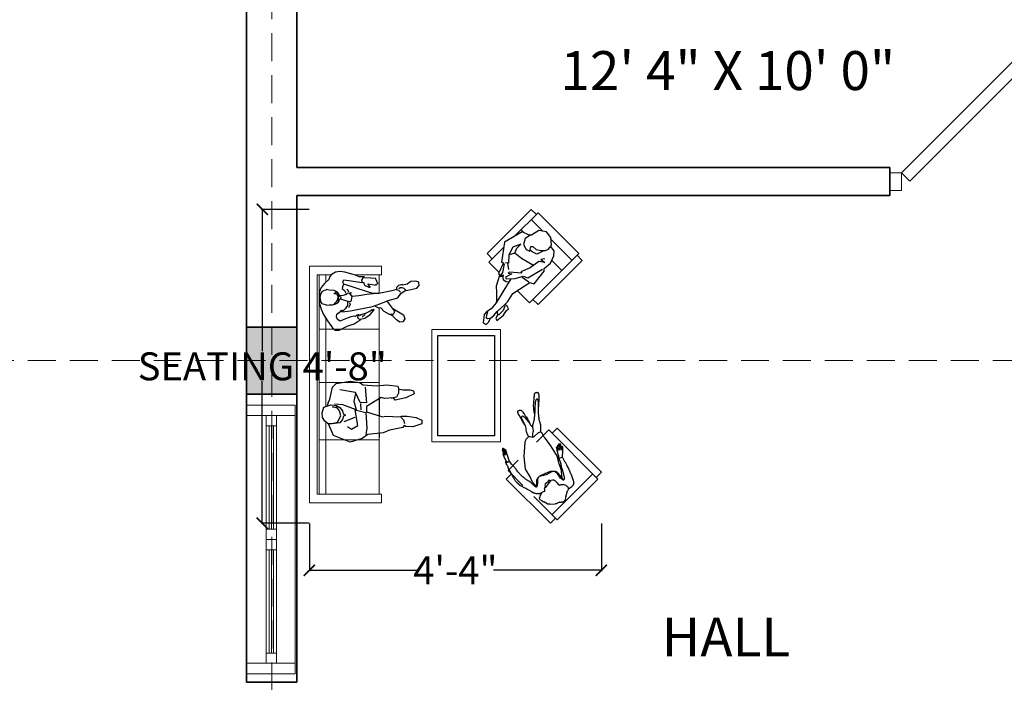
# Model space of a CAD drawing. Units: inches. Extents: x 782 to 2660, y -1008 to 166.
# Tile 7 of 12: x 1058 to 1234, y -176 to -58. Entities that reach past the tile are written whole.
import ezdxf

# ---------------------------------------------------------------- set-up
doc = ezdxf.new("R2010")
doc.units = ezdxf.units.IN
doc.header["$MEASUREMENT"] = 0
doc.linetypes.add('DASHED', pattern=[0.75, 0.5, -0.25])
for name, color, linetype, lineweight in [('A-ANNO-DIMS', 4, 'Continuous', 18), ('A-AREA-IDEN', 4, 'Continuous', 18), ('A-COLS', 7, 'Continuous', 35), ('A-Door', 150, 'Continuous', 18), ('A-FURN', 8, 'Continuous', 13), ('A-Glaz', 4, 'Continuous', 18), ('A-GRID', 8, 'DASHED', 13), ('A-WALL', 7, 'Continuous', 35)]:
    doc.layers.add(name, color=color, linetype=linetype, lineweight=lineweight)
doc.layers.add('NET 01', color=8, linetype='Continuous')
doc.layers.add('NOITHAT', color=21, linetype='Continuous')
doc.styles.get("Standard").update_dxf_attribs({"font": 'arial.ttf'})
doc.dimstyles.get("Standard").update_dxf_attribs({"dimtxt": 5, "dimasz": 2, "dimexe": 0.18, "dimexo": 0.0625, "dimgap": 0.09, "dimtad": 0, "dimtih": 1, "dimtoh": 1, "dimdec": 0, "dimzin": 0, "dimdsep": 46, "dimlunit": 3, "dimtxsty": 'Standard', "dimblk": 'ARCHTICK', "dimcen": 0.09, "dimadec": 0, "dimazin": 0, "dimtfac": 1, "dimtdec": 0, "dimtofl": 0, "dimtmove": 0, "dimatfit": 3, "dimfxl": 1, "dimtolj": 1, "dimtzin": 0, "dimarcsym": 0})

# ---------------------------------------------------------------- blocks, each defined once
blk = doc.blocks.new('A$C592222DF')
at = {"layer": 'A-Door'}
for points in [[(-0.0354, -0.0354), (-0.6718, 0.601), (-0.6364, 0.6364), (0, 0)], [(-0.95, 0), (-0.95, -0.075), (-0.9, -0.075), (-0.9, 0)], [(0, 0), (0, -0.075), (0.05, -0.075), (0.05, 0)]]:
    blk.add_lwpolyline(points, close=True, dxfattribs=at)
at = {"layer": 'NET 01'}
blk.add_arc((0, 0), 0.9, 135, 180, dxfattribs=at)
blk = doc.blocks.new('02PFMA09')
at = {"color": 0, "linetype": 'ByBlock'}
for p, q in [((3.05, 8.92), (3.14, 9)), ((3.13, 7.43), (3.05, 8.92)), ((3.14, 9), (3.16, 8.93)), ((5.73, 9.76), (5.71, 9.77)), ((5.73, 9.76), (5.72, 9.77)), ((-13.1, 3.75), (-12.15, 4.37)), ((-12.31, 4.26), (-10.34, 5.72)), ((-10.32, 5.71), (-10.21, 5.9)), ((-9.79, 6.26), (-10.21, 5.9)), ((-9.79, 6.35), (-9.8, 6.25)), ((-8.24, 6.17), (-8.66, 6.39)), ((-8.12, 6.08), (-8.24, 6.17)), ((-8.12, 6.08), (-7.24, 4.99)), ((-7.02, 3.76), (-7.02, 4.36)), ((-4.78, 5.75), (-5.53, 5.7)), ((-4.02, 5.38), (-5.5, 5.67)), ((-4.78, 5.75), (-2.07, 6.47)), ((-2.3, 4.9), (-4.02, 5.38)), ((-2.4, 4.61), (-1.25, 4.02)), ((-2.3, 4.9), (-2.23, 4.9)), ((0.87, 6.65), (-2.07, 6.47)), ((-1.29, 4.26), (-1.18, 3.98)), ((0.87, 6.65), (3.72, 7.15)), ((3.13, 7.43), (3.55, 7.64)), ((3.55, 7.64), (3.51, 7.76)), ((9.01, 6.24), (4.07, 7.14)), ((13.28, 5.24), (9.01, 6.24)), ((13.28, 5.24), (15.05, 5.1)), ((15.45, 4.82), (15.72, 4.28)), ((15.49, 4.74), (18.19, 5.91)), ((18.19, 5.91), (20.99, 6.15)), ((21.57, 4.27), (19.72, 2.97)), ((23.19, 6.75), (20.99, 6.15)), ((23.07, 5.07), (21.57, 4.27)), ((23.85, 5.5), (23.07, 5.07)), ((24.19, 7.17), (23.19, 6.75)), ((24.19, 7.17), (24.32, 7.29)), ((-13.7, 2), (-13.76, 2.21)), ((-13.66, 2.99), (-13.41, 3.42)), ((-13.36, 1.1), (-13.36, -0.48)), ((-6.7, 3.3), (-6.6, 3.26)), ((-5.84, 3.17), (-6.6, 3.26)), ((-5.84, 3.17), (-5.39, 2.98)), ((-4.55, 2.65), (-5.39, 2.98)), ((-4.85, -0.2), (-3.86, 1.35)), ((-4.08, 0.8), (-4.09, 0.98)), ((-3.5, 0.53), (-4.08, 0.8)), ((-3.5, 0.16), (-4.08, -0.2)), ((-3.86, 1.35), (-3.92, 1.85)), ((-3.5, 0.53), (-3.5, 0.16)), ((-0.77, 3.02), (-1.15, 0.28)), ((-1.15, 0.28), (-0.77, -2.45)), ((-0.6, 2.93), (-0.76, 3.23)), ((-0.48, -1.9), (-0.48, 2.46)), ((14.87, 1.49), (15.75, 3.89)), ((15.65, 0.15), (14.96, 1)), ((15.04, 0.89), (15.44, 1.22)), ((15.44, 1.22), (16.2, 1.52)), ((16.2, 1.52), (16.89, 2)), ((18.39, 2.4), (16.89, 2)), ((18.39, 2.4), (19.72, 2.97)), ((20.04, 0.06), (20.17, 0.06)), ((20.17, 0.06), (20.79, -0.03)), ((-12.58, -2.84), (-13.3, -0.82)), ((-12.58, -2.84), (-12.41, -3.29)), ((-12.07, -3.74), (-10.72, -4.74)), ((-7, -3.4), (-7.02, -4.02)), ((-6.6, -2.66), (-6.77, -2.66)), ((-6.03, -2.48), (-6.6, -2.66)), ((-6.03, -2.48), (-5.6, -2.2)), ((-5.6, -2.2), (-5.44, -1.42)), ((-5.29, -1.93), (-5.55, -1.94)), ((-5.44, -1.42), (-4.85, -0.2)), ((-4.71, -1.75), (-5.29, -1.93)), ((-4.34, -1.47), (-4.71, -1.75)), ((-4.08, -0.2), (-4.34, -1.47)), ((-1.19, -3.54), (-1.1, -3.36)), ((-0.73, -2.64), (-0.59, -2.36)), ((9.01, -5.17), (14.26, -2.61)), ((14.4, -2.51), (15.2, -1.7)), ((15.73, -0.33), (15.32, -1.51)), ((-10.25, -5.27), (-10.43, -5.08)), ((-10.21, -5.2), (-10.25, -5.27)), ((-9.79, -5.57), (-10.21, -5.2)), ((-8.24, -5.48), (-8.66, -5.7)), ((-8.12, -5.39), (-8.24, -5.48)), ((-7.02, -4.02), (-8.12, -5.39)), ((-2.07, -5.87), (-4.12, -5.33)), ((-3.98, -5.05), (-4.11, -5.05)), ((-3.98, -5.05), (-2.34, -4.32)), ((-2.34, -4.32), (-1.65, -3.99)), ((-2.07, -5.87), (0.87, -6.06)), ((0.87, -6.06), (3.67, -6.54)), ((4.11, -6.52), (9.01, -5.17)), ((12.6, -12.12), (12.56, -12.13))]:
    blk.add_line(p, q, dxfattribs=at)
blk.add_line((0, 0), (0, 0))
for points in [[(3.14, 9), (2.51, 9.01), (2.01, 9.04), (1.62, 9.06), (1.33, 9.1), (1.12, 9.13), (0.97, 9.16), (0.87, 9.2), (0.79, 9.23), (0.73, 9.25), (0.67, 9.28), (0.6, 9.3), (0.5, 9.31), (0.37, 9.33), (0.19, 9.35), (-0.05, 9.36), (-0.35, 9.38), (-0.73, 9.41), (-1.17, 9.43), (-1.65, 9.46), (-2.15, 9.49), (-2.66, 9.51), (-3.14, 9.54), (-3.59, 9.56), (-3.97, 9.57), (-4.29, 9.59), (-4.53, 9.6), (-4.72, 9.6), (-4.87, 9.6), (-4.98, 9.6), (-5.08, 9.6), (-5.16, 9.59), (-5.25, 9.59), (-5.35, 9.58), (-5.45, 9.57), (-5.57, 9.56), (-5.69, 9.55), (-5.82, 9.54), (-5.94, 9.54), (-6.06, 9.53), (-6.18, 9.52), (-6.29, 9.51), (-6.39, 9.51), (-6.48, 9.5), (-6.56, 9.5), (-6.64, 9.5), (-6.7, 9.49), (-6.76, 9.49), (-6.81, 9.49), (-6.86, 9.49), (-6.89, 9.49), (-6.93, 9.49), (-6.96, 9.49), (-7, 9.49), (-7.05, 9.48), (-7.1, 9.48), (-7.16, 9.47), (-7.24, 9.46), (-7.32, 9.45), (-7.42, 9.44), (-7.51, 9.43), (-7.61, 9.42), (-7.7, 9.4), (-7.79, 9.39), (-7.87, 9.38), (-7.93, 9.37), (-7.99, 9.36), (-8.03, 9.35), (-8.07, 9.34), (-8.11, 9.33), (-8.14, 9.32), (-8.17, 9.31), (-8.21, 9.3), (-8.25, 9.29), (-8.3, 9.27), (-8.35, 9.25), (-8.42, 9.22), (-8.49, 9.18), (-8.57, 9.12), (-8.66, 9.05), (-8.77, 8.97), (-8.89, 8.86), (-9.02, 8.72), (-9.16, 8.53), (-9.3, 8.27), (-9.43, 7.94), (-9.56, 7.52), (-9.68, 6.99), (-9.79, 6.35)], [(5.68, 9.76), (5.96, 9.86), (6.2, 9.95), (6.4, 10.04), (6.57, 10.11), (6.71, 10.18), (6.83, 10.24), (6.92, 10.29), (6.99, 10.34), (7.03, 10.38), (7.07, 10.41), (7.09, 10.44), (7.09, 10.47), (7.09, 10.49), (7.08, 10.5), (7.06, 10.52), (7.04, 10.53), (7.01, 10.54), (6.99, 10.55), (6.95, 10.55), (6.9, 10.55), (6.83, 10.54), (6.74, 10.52), (6.63, 10.49), (6.49, 10.45), (6.32, 10.4), (6.13, 10.34), (5.91, 10.27), (5.69, 10.19), (5.46, 10.1), (5.22, 10.01), (5, 9.91), (4.79, 9.8), (4.59, 9.7), (4.41, 9.59), (4.23, 9.48), (4.04, 9.36), (3.84, 9.25), (3.61, 9.13), (3.35, 9.01), (3.05, 8.89)], [(3.12, 7.71), (3.95, 7.81), (4.67, 7.89), (5.29, 7.97), (5.81, 8.04), (6.25, 8.1), (6.61, 8.15), (6.9, 8.2), (7.14, 8.25), (7.32, 8.29), (7.47, 8.33), (7.57, 8.36), (7.65, 8.4), (7.69, 8.43), (7.72, 8.46), (7.73, 8.49), (7.73, 8.52), (7.72, 8.55), (7.7, 8.57), (7.65, 8.59), (7.56, 8.62), (7.43, 8.63), (7.25, 8.65), (7, 8.66), (6.68, 8.66)], [(6.02, 8.53), (6.72, 8.67), (7.25, 8.79), (7.63, 8.89), (7.88, 8.96), (8.03, 9.02), (8.1, 9.07), (8.12, 9.11), (8.12, 9.15), (8.1, 9.18), (8.08, 9.2), (8.04, 9.23), (7.97, 9.25), (7.87, 9.26), (7.73, 9.26), (7.54, 9.25), (7.3, 9.23)], [(7.19, 9.74), (7.59, 9.77), (7.9, 9.78), (8.12, 9.78), (8.28, 9.77), (8.38, 9.76), (8.44, 9.74), (8.47, 9.71), (8.49, 9.68), (8.49, 9.64), (8.46, 9.6), (8.38, 9.55), (8.2, 9.48), (7.91, 9.39), (7.47, 9.28), (6.86, 9.14), (6.05, 8.97)], [(6.49, 10.05), (7.06, 10.13), (7.49, 10.19), (7.8, 10.22), (8.02, 10.24), (8.16, 10.23), (8.24, 10.22), (8.28, 10.19), (8.29, 10.16), (8.3, 10.13), (8.27, 10.09), (8.19, 10.04), (8.04, 9.97), (7.77, 9.89), (7.37, 9.79), (6.82, 9.67), (6.08, 9.51)], [(23.49, 5.3), (23.63, 5.3), (23.83, 5.32), (24.11, 5.37), (24.43, 5.44), (24.81, 5.53), (25.24, 5.66), (25.7, 5.81), (26.19, 5.99), (26.71, 6.21), (27.25, 6.45), (27.78, 6.7), (28.3, 6.96), (28.8, 7.22), (29.26, 7.46), (29.68, 7.68), (30.03, 7.88), (30.31, 8.03), (30.52, 8.15), (30.68, 8.25), (30.8, 8.32), (30.87, 8.38), (30.92, 8.42), (30.95, 8.46), (30.97, 8.51), (30.99, 8.56), (31, 8.62), (31.02, 8.68), (31.03, 8.75), (31.04, 8.82), (31.05, 8.9), (31.05, 8.98), (31.05, 9.06), (31.05, 9.14), (31.04, 9.22), (31.02, 9.3), (31, 9.38), (30.97, 9.45), (30.93, 9.52), (30.88, 9.58), (30.82, 9.64), (30.75, 9.69), (30.67, 9.73), (30.58, 9.76), (30.47, 9.77), (30.36, 9.78), (30.23, 9.78), (30.1, 9.77), (29.95, 9.74), (29.78, 9.7), (29.57, 9.64), (29.27, 9.52), (28.86, 9.35), (28.29, 9.1), (27.53, 8.76), (26.55, 8.31), (25.31, 7.73)], [(24.32, 7.29), (25.49, 7.8), (26.4, 8.17), (27.09, 8.42), (27.59, 8.56), (27.94, 8.62), (28.17, 8.61), (28.31, 8.56), (28.39, 8.48), (28.45, 8.38), (28.48, 8.28), (28.47, 8.17), (28.43, 8.05), (28.34, 7.91), (28.2, 7.76), (28.01, 7.6), (27.77, 7.42), (27.46, 7.22), (27.08, 7.01), (26.66, 6.78), (26.18, 6.54), (25.66, 6.29), (25.09, 6.04), (24.48, 5.77), (23.85, 5.5)], [(20.79, -0.03), (22.71, -0.38), (24.15, -0.61), (25.2, -0.75), (25.92, -0.81), (26.37, -0.82), (26.62, -0.77), (26.73, -0.7), (26.78, -0.63), (26.82, -0.56), (26.85, -0.5), (26.88, -0.45), (26.91, -0.4), (26.94, -0.35), (26.96, -0.29), (26.97, -0.23), (26.98, -0.17), (26.98, -0.09), (26.98, -0.01), (26.96, 0.08), (26.95, 0.17), (26.93, 0.27), (26.9, 0.36), (26.88, 0.45), (26.85, 0.54), (26.82, 0.62), (26.78, 0.69), (26.7, 0.77), (26.57, 0.84), (26.39, 0.92), (26.12, 1.01), (25.77, 1.11), (25.3, 1.23), (24.72, 1.36), (24.05, 1.5), (23.31, 1.64), (22.54, 1.76), (21.77, 1.87), (21.02, 1.96), (20.33, 2), (19.74, 2.01)], [(20.17, 0.06), (21.44, -0.08), (22.42, -0.16), (23.16, -0.19), (23.69, -0.17), (24.04, -0.11), (24.25, -0.02), (24.36, 0.09), (24.4, 0.22), (24.41, 0.36), (24.34, 0.5), (24.16, 0.67), (23.83, 0.86), (23.3, 1.09), (22.54, 1.35), (21.5, 1.66), (20.21, 2)], [(-1.25, -3.45), (-1.62, -3.66), (-1.92, -3.82), (-2.16, -3.95), (-2.36, -4.05), (-2.52, -4.12), (-2.66, -4.18), (-2.79, -4.23), (-2.93, -4.29), (-3.08, -4.36), (-3.24, -4.44), (-3.4, -4.53), (-3.56, -4.62), (-3.72, -4.71), (-3.86, -4.81), (-3.98, -4.91), (-4.07, -5), (-4.13, -5.09), (-4.16, -5.17), (-4.15, -5.25), (-4.12, -5.33), (-4.06, -5.41), (-3.96, -5.49), (-3.84, -5.57), (-3.69, -5.66), (-3.51, -5.74), (-3.3, -5.84), (-3.08, -5.94), (-2.83, -6.05), (-2.57, -6.16), (-2.3, -6.29), (-2.02, -6.43), (-1.74, -6.58), (-1.45, -6.75), (-1.17, -6.93), (-0.89, -7.11), (-0.62, -7.3), (-0.37, -7.47), (-0.13, -7.64), (0.08, -7.79), (0.28, -7.92), (0.44, -8.03), (0.58, -8.11), (0.7, -8.17), (0.8, -8.22), (0.88, -8.26), (0.95, -8.29), (1.01, -8.32), (1.07, -8.34), (1.12, -8.37), (1.17, -8.4), (1.22, -8.44), (1.29, -8.49), (1.37, -8.54), (1.47, -8.6), (1.59, -8.67), (1.74, -8.76), (1.93, -8.85), (2.14, -8.96), (2.38, -9.07), (2.65, -9.19), (2.95, -9.32), (3.27, -9.44), (3.61, -9.56), (3.97, -9.68), (4.35, -9.79), (4.74, -9.9), (5.14, -10), (5.53, -10.09), (5.91, -10.19), (6.27, -10.28), (6.6, -10.38), (6.9, -10.48), (7.16, -10.58), (7.4, -10.69), (7.64, -10.8), (7.91, -10.91), (8.21, -11.02), (8.58, -11.12), (9.04, -11.23), (9.6, -11.34)], [(-7.02, -4.02), (-7.07, -4.21), (-7.11, -4.36), (-7.13, -4.47), (-7.15, -4.55), (-7.15, -4.62), (-7.15, -4.68), (-7.15, -4.75), (-7.15, -4.82), (-7.14, -4.91), (-7.13, -5.01), (-7.12, -5.13), (-7.1, -5.26), (-7.07, -5.4), (-7.03, -5.55), (-6.98, -5.71), (-6.91, -5.87), (-6.82, -6.04), (-6.72, -6.21), (-6.6, -6.37), (-6.48, -6.53), (-6.36, -6.68), (-6.23, -6.83), (-6.11, -6.97), (-5.99, -7.09), (-5.89, -7.2), (-5.78, -7.3), (-5.68, -7.39), (-5.58, -7.48), (-5.47, -7.57), (-5.35, -7.67), (-5.21, -7.78), (-5.05, -7.89), (-4.87, -8.03), (-4.67, -8.18), (-4.45, -8.34), (-4.21, -8.52), (-3.96, -8.71), (-3.7, -8.92), (-3.43, -9.13), (-3.15, -9.35), (-2.88, -9.58), (-2.6, -9.82), (-2.33, -10.05), (-2.07, -10.27), (-1.82, -10.49), (-1.59, -10.68), (-1.38, -10.85), (-1.19, -10.99), (-1.03, -11.11), (-0.89, -11.19), (-0.78, -11.25), (-0.68, -11.29), (-0.59, -11.32), (-0.51, -11.34), (-0.42, -11.36), (-0.34, -11.39), (-0.25, -11.42), (-0.15, -11.47), (-0.05, -11.51), (0.06, -11.57), (0.18, -11.63), (0.3, -11.69), (0.43, -11.75), (0.57, -11.81), (0.71, -11.87), (0.86, -11.93), (1.03, -11.98), (1.22, -12.04), (1.45, -12.09), (1.7, -12.15), (2, -12.2), (2.35, -12.25), (2.74, -12.3), (3.17, -12.35), (3.63, -12.4), (4.09, -12.45), (4.55, -12.49), (4.99, -12.53), (5.4, -12.57), (5.77, -12.61), (6.08, -12.64), (6.33, -12.67), (6.54, -12.7), (6.7, -12.72), (6.84, -12.74), (6.95, -12.75), (7.04, -12.76), (7.13, -12.76), (7.2, -12.76), (7.28, -12.76), (7.35, -12.75), (7.42, -12.74), (7.49, -12.73), (7.55, -12.72), (7.62, -12.71), (7.69, -12.7), (7.75, -12.7), (7.84, -12.7), (7.97, -12.71), (8.15, -12.72), (8.4, -12.75), (8.75, -12.79), (9.21, -12.84), (9.8, -12.91)], [(10, -12.41), (9.95, -12.7), (9.89, -12.86), (9.81, -12.9), (9.74, -12.85), (9.67, -12.74), (9.61, -12.57), (9.56, -12.38), (9.53, -12.18), (9.51, -12), (9.52, -11.84), (9.54, -11.7), (9.57, -11.58), (9.6, -11.49), (9.63, -11.41), (9.65, -11.37), (9.66, -11.35)], [(12.73, -11.52), (13.36, -11.44), (13.82, -11.38), (14.16, -11.33), (14.38, -11.3), (14.51, -11.27), (14.57, -11.24), (14.59, -11.22), (14.59, -11.21), (14.58, -11.19), (14.58, -11.17), (14.57, -11.15), (14.57, -11.13), (14.56, -11.12), (14.55, -11.1), (14.54, -11.09), (14.53, -11.07), (14.51, -11.06), (14.48, -11.06), (14.44, -11.05), (14.39, -11.05), (14.32, -11.05), (14.23, -11.06), (14.12, -11.06), (13.98, -11.07), (13.82, -11.09), (13.62, -11.1), (13.41, -11.12), (13.19, -11.14), (12.95, -11.16), (12.71, -11.18), (12.47, -11.2), (12.24, -11.22), (12.03, -11.25), (11.82, -11.27), (11.63, -11.29), (11.44, -11.31), (11.27, -11.33), (11.12, -11.34), (10.97, -11.35), (10.84, -11.36), (10.71, -11.36), (10.6, -11.37), (10.48, -11.37), (10.35, -11.37), (10.2, -11.38), (10.04, -11.4), (9.84, -11.42), (9.61, -11.46)], [(14.99, -11.92), (15.09, -11.9), (15.17, -11.88), (15.23, -11.85), (15.27, -11.83), (15.3, -11.8), (15.32, -11.77), (15.32, -11.74), (15.32, -11.71), (15.32, -11.67), (15.28, -11.64), (15.18, -11.62), (14.99, -11.61), (14.67, -11.61), (14.2, -11.64), (13.54, -11.7), (12.67, -11.79)], [(14.99, -11.54), (14.99, -11.51), (14.96, -11.47), (14.88, -11.43), (14.71, -11.4), (14.44, -11.39), (14.04, -11.4), (13.48, -11.44), (12.73, -11.52)], [(9.56, -12.39), (9.77, -12.4), (9.94, -12.41), (10.08, -12.42), (10.2, -12.44), (10.3, -12.45), (10.39, -12.47), (10.46, -12.48), (10.52, -12.49), (10.58, -12.5), (10.64, -12.51), (10.7, -12.51), (10.76, -12.52), (10.82, -12.53), (10.89, -12.53), (10.97, -12.54), (11.05, -12.54), (11.13, -12.55), (11.23, -12.56), (11.33, -12.58), (11.43, -12.59), (11.52, -12.6), (11.61, -12.61), (11.7, -12.62), (11.77, -12.62), (11.83, -12.62), (11.89, -12.62), (11.93, -12.62), (11.97, -12.62), (12.01, -12.61), (12.05, -12.61), (12.1, -12.6), (12.14, -12.6), (12.2, -12.59), (12.27, -12.59), (12.34, -12.59), (12.41, -12.58), (12.48, -12.58), (12.55, -12.58), (12.61, -12.58), (12.67, -12.59), (12.73, -12.59), (12.77, -12.59), (12.81, -12.59), (12.85, -12.6), (12.88, -12.6), (12.92, -12.6), (12.95, -12.61), (12.99, -12.61), (13.03, -12.62), (13.07, -12.62), (13.11, -12.62), (13.15, -12.62), (13.18, -12.61), (13.21, -12.6), (13.23, -12.59), (13.24, -12.56), (13.24, -12.53), (13.21, -12.49), (13.17, -12.45), (13.11, -12.39), (13.02, -12.34), (12.89, -12.27), (12.74, -12.2), (12.54, -12.13)], [(13.04, -12.35), (13.55, -12.31), (14.08, -12.26), (14.46, -12.21), (14.72, -12.18), (14.87, -12.14), (14.95, -12.11), (14.98, -12.08), (14.99, -12.04), (14.98, -12.01), (14.95, -11.98), (14.86, -11.96), (14.69, -11.94), (14.4, -11.95), (13.98, -11.98), (13.38, -12.03), (12.6, -12.12)]]:
    blk.add_lwpolyline(points, dxfattribs=at)
blk.add_lwpolyline([(3.13, 7.43), (2.49, 7.44), (1.98, 7.44), (1.59, 7.44), (1.3, 7.43), (1.09, 7.42), (0.94, 7.4), (0.83, 7.38), (0.74, 7.36), (0.65, 7.33), (0.54, 7.3), (0.42, 7.27), (0.28, 7.24), (0.09, 7.2), (-0.13, 7.16), (-0.4, 7.12), (-0.73, 7.07), (-1.11, 7.03), (-1.55, 6.98), (-2.02, 6.93), (-2.5, 6.88), (-2.97, 6.83), (-3.43, 6.78), (-3.85, 6.74), (-4.21, 6.69), (-4.51, 6.65), (-4.74, 6.61), (-4.93, 6.57), (-5.06, 6.53), (-5.17, 6.49), (-5.24, 6.46), (-5.3, 6.42), (-5.35, 6.38), (-5.41, 6.34), (-5.46, 6.29), (-5.51, 6.25), (-5.55, 6.2), (-5.59, 6.16), (-5.63, 6.11), (-5.66, 6.07), (-5.68, 6.03), (-5.69, 5.99), (-5.69, 5.95), (-5.68, 5.92), (-5.67, 5.88), (-5.64, 5.83), (-5.6, 5.79), (-5.56, 5.73), (-5.5, 5.67), (-5.43, 5.6), (-5.33, 5.51), (-5.16, 5.41), (-4.9, 5.3), (-4.52, 5.16), (-4, 5), (-3.3, 4.82), (-2.4, 4.61)])
for centre, radius, start, end in [((-9.13, 5.51), 1, 62.007, 131.0995), ((-8.02, 4.36), 1, 0, 38.6768), ((-2.23, 3.9), 1, 21.2691, 90), ((-1.76, 3.16), 1, 351.9817, 59.8215), ((3.89, 6.16), 1, 79.664, 99.8193), ((15.01, 4.6), 0.5, 26.6038, 85.4677), ((15.28, 4.06), 0.5, 340.0861, 26.6038), ((-12.8, 2.48), 1, 149.5843, 195.8839), ((-12.74, 2.28), 1, 195.8839, 215.9577), ((-14.36, 1.1), 1, 0, 35.9577), ((-12.54, 2.92), 1, 123.5157, 149.5843), ((-6.52, 3.76), 0.5, 180, 249.0498), ((-4.92, 1.72), 1, 7.286, 68.641), ((-1.48, 2.46), 1, 0, 28.4429), ((15.34, 1.32), 0.5, 160.0861, 218.8571), ((15.26, -0.17), 0.5, 340.8781, 38.8571), ((-12.36, -0.48), 1, 180, 199.5267), ((-11.48, -2.94), 1, 200.5274, 233.5498), ((-6.27, -3.21), 0.747, 131.875, 194.63), ((-2.09, -3.09), 1, 295.9892, 332.9967), ((-1.76, -2.58), 1, 300.1785, 8.0241), ((-1.48, -1.9), 1, 332.8271, 0), ((14.04, -2.16), 0.5, 296.0412, 315.1007), ((14.85, -1.35), 0.5, 315.1007, 340.8781), ((-11.32, -5.55), 1, 27.9198, 53.5498), ((-9.13, -4.82), 1, 228.8141, 298.1014), ((3.84, -5.56), 1, 260.2266, 285.378)]:
    blk.add_arc(centre, radius, start, end, dxfattribs=at)
for centre, radius, start, end in [((16.79, 9.1), 9.61, 263.4345, 289.7848), ((0.77, -27.9), 35.41, 57.624, 59.3879), ((9.55, -11.79), 0.45, 53.8302, 82.9173)]:
    blk.add_arc(centre, radius, start, end)
blk = doc.blocks.new('A$C7E2525C2')
for p, q in [((2190.1, 2433.4), (1822.4, 2065.8)), ((1836.5, 1995.1), (2246.7, 2405.1)), ((2232.6, 2391), (2190.1, 2433.4)), ((2246.7, 2405.1), (2586, 2065.6)), ((2203.8, 2362.2), (2543.1, 2022.7)), ((367.6, 2245.4), (28.3, 1906)), ((777.8, 1835.4), (367.6, 2245.4)), ((424.2, 2273.7), (381.8, 2231.3)), ((791.9, 1906.1), (424.2, 2273.7)), ((424.2, 2188.9), (249, 2013.6)), ((425.7, 2020.6), (509.1, 2104)), ((1822.4, 2065.8), (1864.8, 2023.3)), ((2586, 2065.6), (2390.7, 1870.4)), ((2614.3, 2009.1), (2571.9, 2051.5)), ((1939.1, 1892.4), (1836.5, 1995.1)), ((2246.6, 1641.4), (2614.3, 2009.1)), ((42.4, 1891.8), (0, 1849.4)), ((28.3, 1906), (223.6, 1710.7)), ((182.1, 1946.7), (84.9, 1849.4)), ((749.5, 1863.7), (791.9, 1906.1)), ((0, 1849.4), (367.8, 1481.8)), ((675.2, 1732.7), (777.8, 1835.4)), ((2175.8, 1655.6), (2089.9, 1741.6)), ((2299.6, 1779.3), (2175.8, 1655.6)), ((2204.1, 1683.9), (2246.6, 1641.4)), ((314.7, 1619.6), (438.5, 1495.9)), ((438.5, 1495.9), (524.4, 1581.9)), ((367.8, 1481.8), (410.2, 1524.2)), ((473.1, 65), (473.1, 600.7)), ((544.5, 600.7), (473.1, 600.7)), ((544.5, 375.6), (544.5, 600.7)), ((544.5, 582.9), (699.7, 582.9)), ((822.4, 582.9), (2372.5, 582.9)), ((996.9, 82.9), (996.9, 582.9)), ((1441.2, 82.9), (1441.2, 582.9)), ((1920.2, 82.9), (1920.2, 582.9)), ((2372.5, 600.7), (2372.5, 65)), ((2372.5, 600.7), (2444, 600.7)), ((2444, 600.7), (2444, 65)), ((544.5, 65), (544.5, 183.6)), ((607.3, 136.4), (544.5, 136.4)), ((2372.5, 82.9), (544.5, 82.9)), ((1641.4, 136.4), (905.1, 136.4)), ((2372.5, 136.4), (1769.1, 136.4)), ((1901.7, 136.4), (1769.1, 136.4))]:
    blk.add_line(p, q)
blk.add_lwpolyline([(1001.5, 1019.5), (1001.5, 1593.7), (1937.2, 1593.7), (1937.2, 1019.5)], close=True)
for points in [[(473.1, 65), (473.1, 0), (2444, 0), (2444, 65)], [(544.5, 65), (2372.5, 65)]]:
    blk.add_lwpolyline(points)
at = {"layer": 'NOITHAT'}
for p, q in [((187.2, 1976.6), (176, 1911.1)), ((233, 2012.4), (187.2, 1976.6)), ((297.3, 2017.2), (233, 2012.4)), ((305.9, 2009.8), (297.3, 2017.2)), ((345.6, 2040.3), (305.9, 2009.8)), ((329.9, 1992.2), (312.6, 2007.1)), ((343, 1967.3), (329.9, 1992.2)), ((387.8, 2038.6), (345.6, 2040.3)), ((446.4, 2010.7), (387.8, 2038.6)), ((490.8, 1957.5), (446.4, 2010.7)), ((176, 1911.1), (214.3, 1852.5)), ((307.4, 1861.2), (334.4, 1889.1)), ((334.4, 1889.1), (340.8, 1933.2)), ((340.8, 1933.2), (343, 1967.3)), ((340.9, 1935.8), (348.4, 1943.3)), ((344.3, 1951.3), (372.6, 1896.8)), ((372.6, 1896.8), (352.9, 1858.2)), ((411.2, 1962.8), (417, 1929.3)), ((417, 1929.3), (442, 1961.9)), ((442, 1961.9), (432.9, 1911.1)), ((432.9, 1911.1), (485.2, 1839.1)), ((513.6, 1956), (490.8, 1957.5)), ((570.6, 1819.7), (496.7, 1943.4)), ((619.9, 1873.5), (513.6, 1956)), ((214.2, 1833.1), (186.3, 1774.4)), ((211.6, 1845.9), (242.6, 1798.1)), ((214.3, 1852.5), (214.2, 1833.1)), ((292, 1785.7), (332.4, 1808.1)), ((308.6, 1845.1), (307.4, 1861.2)), ((348, 1836.8), (308.6, 1845.1)), ((332.4, 1808.1), (348, 1836.8)), ((352.9, 1858.2), (338, 1840.9)), ((464, 1863.3), (409.7, 1768.7)), ((485.2, 1839.1), (520, 1762.5)), ((555.6, 1783), (570.6, 1819.7)), ((605.5, 1828.8), (567.6, 1774.2)), ((609.6, 1838.8), (619.9, 1873.5)), ((663.1, 1750.7), (609.6, 1838.8)), ((169.7, 1764.6), (192.3, 1787.2)), ((186.3, 1774.4), (273.3, 1625.8)), ((242.6, 1798.1), (292, 1785.7)), ((323.7, 1729.9), (290.5, 1762.9)), ((290.5, 1762.9), (313.4, 1695.1)), ((363.7, 1713.5), (323.7, 1729.9)), ((409.7, 1768.7), (363.7, 1713.5)), ((520, 1762.5), (530.8, 1769.8)), ((530.8, 1769.8), (522.5, 1664.1)), ((575.2, 1716.5), (555.6, 1783)), ((699.4, 1696.8), (663.1, 1750.7)), ((313.4, 1695.1), (377.3, 1661.2)), ((363.7, 1713.5), (378.7, 1664.5)), ((377.3, 1661.2), (446.9, 1660)), ((446.9, 1660), (444, 1633.9)), ((447.5, 1651.9), (501.8, 1660.9)), ((522.5, 1664.1), (531.2, 1656.6)), ((531.2, 1656.6), (535.4, 1686.1)), ((535.4, 1686.1), (565.1, 1635)), ((579.2, 1640.9), (575.2, 1716.5)), ((579.5, 1679.7), (672.7, 1622.1)), ((605.4, 1657.4), (601.9, 1639.4)), ((767.3, 1653.5), (699.4, 1696.8)), ((791.9, 1627.9), (767.3, 1653.5)), ((804.7, 1649.9), (791.9, 1627.9)), ((827.6, 1660.8), (804.7, 1649.9)), ((844.2, 1641.5), (827.6, 1660.8)), ((881.4, 1618.5), (844.2, 1641.5)), ((273.3, 1625.8), (438.4, 1601.1)), ((438.4, 1601.1), (445.2, 1617.8)), ((445.2, 1617.8), (533.9, 1577.6)), ((524.8, 1612.5), (452.6, 1626.5)), ((558.7, 1590.8), (524.8, 1612.5)), ((533.9, 1577.6), (541.3, 1586.3)), ((541.3, 1586.3), (638.7, 1558.1)), ((546.9, 1619), (561.5, 1597.5)), ((565, 1615.6), (546.9, 1619)), ((561.5, 1597.5), (558.7, 1590.8)), ((589.1, 1617.4), (565, 1615.6)), ((565.1, 1635), (579.2, 1640.9)), ((601.9, 1639.4), (589.1, 1617.4)), ((638.7, 1558.1), (690.3, 1560.4)), ((672.7, 1622.1), (778.2, 1556.4)), ((690.3, 1560.4), (759.9, 1559.2)), ((759.9, 1559.2), (777.9, 1555.7)), ((791.9, 1627.9), (851.6, 1564.5)), ((804.6, 1630.4), (841.3, 1615.4)), ((841.3, 1615.4), (879.7, 1576.3)), ((851.6, 1564.5), (880.4, 1568.3)), ((886.1, 1534.8), (851.6, 1564.5)), ((880.4, 1568.3), (905.7, 1554)), ((924.2, 1561.1), (881.4, 1618.5)), ((905.7, 1554), (924.2, 1561.1)), ((777.9, 1555.7), (827.7, 1515.8)), ((827.7, 1515.8), (842.3, 1494.3)), ((879, 1479.3), (840.9, 1490.9)), ((842.3, 1494.3), (853.7, 1477)), ((905, 1476.4), (879, 1479.3)), ((907.3, 1510.5), (886.1, 1534.8)), ((912.5, 1485), (905, 1476.4)), ((937.2, 1495.3), (907.3, 1510.5)), ((907.9, 1502.5), (912.5, 1485)), ((958.5, 1474), (937.2, 1495.3)), ((853.7, 1477), (874.1, 1457.9)), ((874.1, 1457.9), (944.3, 1448.6)), ((944.3, 1448.6), (958.5, 1474)), ((606.9, 912.3), (597.2, 888.1)), ((632.6, 913.9), (606.9, 912.3)), ((655.9, 896.1), (632.6, 913.9)), ((1732.9, 889.2), (1755.5, 938.1)), ((1755.5, 938.1), (1785.6, 938.1)), ((1785.6, 938.1), (1811.9, 862.9)), ((597.2, 888.1), (600.4, 844.6)), ((600.4, 844.6), (621.4, 814)), ((672.9, 820.5), (655.9, 896.1)), ((1503.2, 836.5), (1510.8, 866.6)), ((1503.2, 780.1), (1503.2, 836.5)), ((1510.8, 866.6), (1537.1, 874.2)), ((1537.1, 874.2), (1571, 802.7)), ((1721.6, 814), (1732.9, 889.2)), ((1811.9, 862.9), (1808.2, 802.7)), ((621.4, 814), (631, 778.5)), ((631, 778.5), (624.6, 772.1)), ((624.6, 772.1), (634.3, 743.1)), ((634.3, 743.1), (650.4, 725.4)), ((658.4, 791.4), (652, 772.1)), ((652, 772.1), (653.6, 757.6)), ((653.6, 757.6), (661.6, 746.3)), ((674.5, 805.9), (658.4, 791.4)), ((674.5, 744.7), (669.7, 730.2)), ((676.1, 797.9), (672.9, 820.5)), ((689, 759.2), (674.5, 744.7)), ((700.3, 762.4), (676.1, 797.9)), ((735.7, 738.3), (700.3, 762.4)), ((827.5, 701.2), (877.4, 785)), ((877.4, 785), (911.2, 794.7)), ((911.2, 794.7), (935.4, 778.5)), ((940.2, 752.8), (920.9, 725.4)), ((935.4, 778.5), (940.2, 752.8)), ((1461.8, 644.7), (1473.1, 738.7)), ((1473.1, 738.7), (1495.7, 742.5)), ((1495.7, 742.5), (1503.2, 780.1)), ((1499.5, 742.5), (1529.6, 742.5)), ((1529.6, 742.5), (1563.5, 727.4)), ((1571, 802.7), (1589.8, 716.2)), ((1721.6, 768.8), (1721.6, 814)), ((1729.1, 757.5), (1721.6, 768.8)), ((1721.6, 633.4), (1729.1, 757.5)), ((1733.7, 765.2), (1753.2, 784.7)), ((1753.2, 784.7), (1782.4, 792.8)), ((1808.2, 802.7), (1800.6, 791.4)), ((1800.6, 791.4), (1815.7, 780.1)), ((1815.7, 780.1), (1838.3, 667.2)), ((650.4, 725.4), (666.5, 725.4)), ((666.5, 725.4), (677.7, 688.3)), ((677.7, 688.3), (700.3, 580.3)), ((759.9, 656.1), (735.7, 738.3)), ((767.9, 648), (822.7, 691.5)), ((822.7, 691.5), (848.4, 710.9)), ((848.4, 710.9), (866.1, 704.4)), ((875.8, 667.3), (851.6, 623.8)), ((866.1, 704.4), (875.8, 694.7)), ((875.8, 694.7), (875.8, 667.3)), ((890.3, 696.3), (877.4, 680.2)), ((920.9, 725.4), (890.3, 696.3)), ((1563.5, 727.4), (1574.8, 682.3)), ((1589.8, 716.2), (1571, 701.1)), ((1571, 701.1), (1574.8, 625.9)), ((1838.3, 667.2), (1860.9, 614.6)), ((700.3, 580.3), (700.3, 530.3)), ((784, 594.8), (759.9, 656.1)), ((809.8, 527.1), (784, 594.8)), ((822.7, 580.3), (809.8, 551.3)), ((851.6, 623.8), (821, 596.4)), ((821, 596.4), (822.7, 580.3)), ((1469.4, 558.2), (1461.8, 644.7)), ((1574.8, 625.9), (1567.2, 599.5)), ((1567.2, 599.5), (1642.5, 475.4)), ((1577.4, 582.9), (1720.6, 582.9)), ((1687.7, 475.4), (1729.1, 610.8)), ((1729.1, 610.8), (1721.6, 633.4)), ((1860.9, 614.6), (1875.9, 486.7)), ((1864.6, 582.9), (1901.7, 582.9)), ((571.4, 511), (569.8, 459.4)), ((574.7, 552.9), (571.4, 511)), ((589.2, 556.1), (574.7, 552.9)), ((594, 561), (589.2, 556.1)), ((603.7, 562.6), (594, 561)), ((611.7, 570.6), (603.7, 562.6)), ((616.5, 573.9), (611.7, 570.6)), ((621.4, 557.7), (616.5, 573.9)), ((619.8, 490.1), (631, 557.7)), ((631, 557.7), (621.4, 557.7)), ((643.9, 507.8), (626.2, 490.1)), ((631, 459.4), (648.7, 496.5)), ((648.7, 506.2), (643.9, 507.8)), ((648.7, 496.5), (648.7, 506.2)), ((700.3, 530.3), (687.4, 483.6)), ((701.9, 533.6), (709.9, 478.8)), ((843.6, 343.4), (809.8, 527.1)), ((837.2, 540), (832.3, 535.2)), ((832.3, 535.2), (843.6, 520.7)), ((843.6, 520.7), (835.5, 522.3)), ((835.5, 522.3), (846.8, 506.2)), ((875.8, 506.2), (837.2, 540)), ((846.8, 506.2), (864.5, 473.9)), ((906.4, 461), (875.8, 506.2)), ((1461.8, 449.1), (1469.4, 558.2)), ((561.8, 414.3), (547.3, 385.3)), ((569.8, 459.4), (561.8, 456.2)), ((561.8, 456.2), (561.8, 414.3)), ((589.2, 436), (565.8, 451.4)), ((603.7, 439.2), (589.2, 436)), ((594, 349.8), (610.1, 436.9)), ((606.9, 451.4), (631, 459.4)), ((610.1, 436.9), (606.9, 451.4)), ((626.2, 490.1), (619.8, 490.1)), ((687.4, 483.6), (621.4, 288.6)), ((709.9, 478.8), (719.6, 411.1)), ((719.6, 411.1), (724.4, 356.3)), ((864.5, 473.9), (871, 456.2)), ((871, 456.2), (872.6, 446.5)), ((872.2, 458.5), (877.1, 462.5)), ((872.6, 446.5), (879, 430.4)), ((885.5, 419.1), (875.8, 412.7)), ((875.8, 412.7), (882.2, 398.2)), ((877.1, 462.5), (882.8, 456.8)), ((879, 430.4), (885.5, 419.1)), ((882.8, 456.8), (890.2, 445.4)), ((890.2, 445.4), (900.8, 441.3)), ((914.4, 425.6), (906.4, 461)), ((916.1, 422.4), (911.2, 409.5)), ((922.5, 424), (914.4, 425.6)), ((935.4, 399.8), (922.5, 424)), ((1431.7, 340), (1443, 419)), ((1443, 419), (1461.8, 449.1)), ((1480.7, 464.1), (1612.4, 475.4)), ((1608.7, 422.7), (1525.8, 385.1)), ((1612.4, 475.4), (1608.7, 422.7)), ((1616.2, 426.5), (1668.9, 430.2)), ((1642.5, 475.4), (1687.7, 475.4)), ((1671.1, 382.2), (1691.5, 471.6)), ((1691.5, 471.6), (1823.2, 479.2)), ((1823.2, 479.2), (1875.9, 471.6)), ((1875.9, 486.7), (1909.8, 441.5)), ((1909.8, 441.5), (1939.9, 340)), ((547.3, 385.3), (521.5, 295)), ((587.6, 287), (594, 349.8)), ((690.6, 328.9), (676.1, 324)), ((711.5, 341.8), (690.6, 348.2)), ((695.4, 332.1), (726, 353.1)), ((697.1, 316), (695.4, 332.1)), ((726, 353.1), (767.9, 346.6)), ((769.5, 330.5), (748.6, 259.6)), ((767.9, 346.6), (769.5, 330.5)), ((774.4, 333.7), (792.1, 340.2)), ((792.1, 340.2), (821, 325.7)), ((851.6, 296.6), (843.6, 343.4)), ((882.2, 398.2), (891.9, 385.3)), ((898.3, 403), (883.9, 407.9)), ((891.9, 385.3), (888.7, 374)), ((888.7, 374), (893.5, 345)), ((893.5, 345), (916.1, 288.6)), ((911.2, 409.5), (898.3, 403)), ((953.1, 372.4), (935.4, 399.8)), ((974, 316), (953.1, 372.4)), ((1450.5, 223.3), (1431.7, 340)), ((1525.8, 385.1), (1503.2, 253.4)), ((1533.4, 385.1), (1597.4, 370.1)), ((1597.4, 370.1), (1670.5, 391)), ((1670.5, 391), (1627.5, 279.8)), ((1800.6, 403.9), (1671.1, 382.2)), ((1765.7, 289), (1732.3, 382.7)), ((1830.8, 351.2), (1800.6, 403.9)), ((1808.2, 317.4), (1830.8, 351.2)), ((1939.9, 340), (1883.5, 200.8)), ((521.5, 295), (516.7, 258)), ((516.7, 258), (521.5, 217.7)), ((606.9, 278.9), (587.6, 287)), ((621.4, 288.6), (606.9, 278.9)), ((623, 283.8), (645.5, 277.3)), ((645.5, 277.3), (660, 274.1)), ((660, 274.1), (674.5, 291.8)), ((676.1, 324), (663.2, 312.8)), ((674.5, 291.8), (697.1, 304.7)), ((706.7, 246.7), (689, 235.4)), ((705.1, 311.2), (697.1, 316)), ((713.2, 282.1), (705.1, 311.2)), ((724.3, 250.1), (706.7, 246.7)), ((716.4, 251.5), (713.2, 282.1)), ((730.9, 264.4), (724.3, 250.1)), ((738.6, 265.5), (730.9, 264.4)), ((747, 251.8), (738.6, 265.5)), ((764.7, 248.3), (747, 251.8)), ((779.2, 237), (764.7, 248.3)), ((769.5, 317.6), (801.7, 317.6)), ((801.7, 317.6), (827.5, 298.3)), ((827.5, 298.3), (843.6, 280.5)), ((840.4, 267.6), (853.3, 270.9)), ((848.4, 261.2), (840.4, 267.6)), ((843.6, 280.5), (842, 274.1)), ((872.6, 229), (848.4, 261.2)), ((853.3, 270.9), (851.6, 296.6)), ((916.1, 288.6), (932.2, 258)), ((932.2, 258), (917.7, 235.4)), ((1006.2, 248.3), (974, 316)), ((1004.6, 214.4), (1006.2, 248.3)), ((1627.5, 279.8), (1622.7, 210.9)), ((1678.2, 250.5), (1655.6, 235.5)), ((1719.6, 261.8), (1678.2, 250.5)), ((1772.3, 235.5), (1719.6, 261.8)), ((521.5, 217.7), (542.5, 185.4)), ((542.5, 185.4), (558.6, 170.9)), ((558.6, 170.9), (584.3, 162.9)), ((672.9, 166.1), (668.1, 143.5)), ((675.6, 207.7), (672.9, 166.1)), ((689, 235.4), (675.6, 207.7)), ((680.7, 216.3), (694.3, 225.8)), ((694.3, 225.8), (699.7, 204)), ((699.7, 204), (703.8, 225.8)), ((700.7, 239.3), (721.3, 244.7)), ((770.7, 243.6), (701.8, 243.6)), ((703.8, 225.8), (716, 234)), ((716, 234), (732.4, 236.7)), ((732.4, 236.7), (755.5, 232.6)), ((755.1, 245.8), (768.1, 239.3)), ((755.5, 232.6), (774.5, 220.4)), ((774.5, 220.4), (785.4, 208.1)), ((787.2, 219.3), (779.2, 237)), ((793.7, 191.9), (787.2, 219.3)), ((795.3, 164.5), (793.7, 191.9)), ((796.9, 140.3), (795.3, 164.5)), ((895.1, 227.3), (872.6, 229)), ((917.7, 235.4), (895.1, 227.3)), ((928.9, 151.6), (986.9, 193.5)), ((986.9, 193.5), (1004.6, 214.4)), ((1480.7, 193.2), (1450.5, 223.3)), ((1582.3, 170.7), (1480.7, 193.2)), ((1612.4, 155.6), (1582.3, 170.7)), ((1647.9, 227.3), (1640, 231.8)), ((1655.6, 235.5), (1644.3, 194.1)), ((1644.3, 194.1), (1647.9, 227.3)), ((1783.6, 190.3), (1772.3, 235.5)), ((1883.5, 200.8), (1785.8, 158.4)), ((1901.7, 243.6), (1900.8, 243.6)), ((584.3, 162.9), (616.5, 125.8)), ((616.5, 125.8), (650.4, 98.4)), ((650.4, 98.4), (684.2, 83.9)), ((668.1, 143.5), (672.9, 138.7)), ((672.9, 138.7), (676.1, 124.2)), ((676.1, 124.2), (685.8, 104.9)), ((684.2, 83.9), (748.6, 80.7)), ((685.8, 104.9), (708.3, 92)), ((708.3, 92), (734.1, 87.1)), ((734.1, 87.1), (763.1, 92)), ((748.6, 80.7), (787.2, 85.5)), ((763.1, 92), (784, 104.9)), ((784, 104.9), (792.1, 130.6)), ((787.2, 85.5), (830.7, 98.4)), ((792.1, 130.6), (793.7, 140.3)), ((793.7, 140.3), (796.9, 140.3)), ((830.7, 98.4), (875.8, 117.7)), ((875.8, 117.7), (928.9, 151.6)), ((1612.4, 155.6), (1633.8, 149.8))]:
    blk.add_line(p, q, dxfattribs=at)
for points in [[(1051.5, 1069.5), (1051.5, 1543.7), (1887.2, 1543.7), (1887.2, 1069.5)], [(1778.4, 253.6), (1787.7, 189.4), (1785.6, 155.6), (1763, 129.3), (1732.9, 110.5), (1695.2, 106.7), (1646.3, 121.8), (1627.5, 178.1), (1634.7, 225.6), (1651.3, 254.6), (1679.2, 275.3), (1702.9, 282.5), (1711.2, 299.1), (1716.4, 299.1), (1723.6, 283.6), (1750.5, 275.3)]]:
    blk.add_lwpolyline(points, close=True, dxfattribs=at)
at = {"layer": 'NOITHAT', "xscale": -20.72890869400127, "yscale": 20.72890869399998, "zscale": 20.72890869399999, "rotation": 22.25669101692736}
blk.add_blockref('02PFMA09', (2192.3, 1959.9), dxfattribs=at)
blk = doc.blocks.new('WIN-48-FRAME-B')
for p, q in [((8.69, 48), (0, 48)), ((0, 48), (0, 46.15)), ((8.69, 48), (0, 48)), ((8.69, 0), (8.69, 48)), ((8.69, 46.15), (8.69, 48)), ((0, 46.15), (8.69, 46.15)), ((0, 46.15), (8.69, 46.15)), ((0, 1.85), (0, 46.15)), ((3.5, 46.15), (3.5, 1.85)), ((5.35, 46.15), (5.35, 1.85)), ((3.5, 44.31), (5.35, 44.31)), ((4.05, 44.31), (4.05, 25.85)), ((4.42, 44.31), (4.42, 25.85)), ((4.79, 44.31), (4.79, 25.85)), ((5.35, 25.85), (3.5, 25.85)), ((5.35, 24), (3.5, 24)), ((5.35, 22.15), (3.5, 22.15)), ((4.05, 3.69), (4.05, 22.15)), ((4.42, 3.69), (4.42, 22.15)), ((4.79, 3.69), (4.79, 22.15)), ((3.5, 3.69), (5.35, 3.69)), ((0, 1.85), (8.69, 1.85)), ((0, 0), (0, 1.85)), ((0, 1.85), (8.69, 1.85)), ((0, 1.85), (8.69, 1.85)), ((8.69, 1.85), (8.69, 0)), ((8.69, 0), (0, 0)), ((0, 0), (8.69, 0))]:
    blk.add_line(p, q)
blk = doc.blocks.new('COL-9X12')
h = blk.add_hatch(color=256)
h.dxf.hatch_style = 1
h.paths.add_polyline_path([(9, 12), (0, 12), (0, 0), (9, 0)])
blk.add_lwpolyline([(0, 12), (9, 12), (9, 0), (0, 0)], close=True)
blk = doc.blocks.new('_ArchTick')
at = {"color": 0, "linetype": 'ByBlock', "const_width": 0.15}
blk.add_lwpolyline([(-0.5, -0.5), (0.5, 0.5)], dxfattribs=at)
blk = doc.blocks.new('*D45')
at = {"layer": 'A-ANNO-DIMS', "color": 0, "lineweight": -2, "transparency": 16777216}
for p, q in [((1109.83, -91.47), (1101.3, -91.47)), ((1101.48, -91.47), (1101.48, -116.83)), ((1101.48, -147.55), (1101.48, -122.18)), ((1109.83, -147.55), (1101.3, -147.55))]:
    blk.add_line(p, q, dxfattribs=at)
at = {"layer": 'Defpoints', "color": 0, "transparency": 16777216}
for p in [(1109.89, -91.47), (1101.48, -147.55), (1109.89, -147.55)]:
    blk.add_point(p, dxfattribs=at)
at = {"layer": 'A-ANNO-DIMS', "color": 0, "lineweight": -2, "transparency": 16777216, "xscale": 2, "yscale": 2, "zscale": 2}
for p, rotation in [((1101.48, -91.47), 90), ((1101.48, -147.55), 270)]:
    blk.add_blockref('_ArchTick', p, dxfattribs=dict(at, rotation=rotation))
at = {"layer": 'A-ANNO-DIMS', "color": 0, "transparency": 16777216, "insert": (1101.48, -119.51), "char_height": 5, "attachment_point": 5}
blk.add_mtext('\\A1;SEATING 4\'-8"', dxfattribs=at)
blk = doc.blocks.new('*D46')
at = {"layer": 'A-ANNO-DIMS', "color": 0, "lineweight": -2, "transparency": 16777216}
for p, q in [((1109.89, -147.61), (1109.89, -156.14)), ((1162.09, -147.61), (1162.09, -156.14)), ((1109.89, -155.96), (1129.16, -155.96)), ((1162.09, -155.96), (1142.83, -155.96))]:
    blk.add_line(p, q, dxfattribs=at)
at = {"layer": 'Defpoints', "color": 0, "transparency": 16777216}
for p in [(1109.89, -147.55), (1162.09, -147.55), (1162.09, -155.96)]:
    blk.add_point(p, dxfattribs=at)
at = {"layer": 'A-ANNO-DIMS', "color": 0, "lineweight": -2, "transparency": 16777216, "xscale": 2, "yscale": 2, "zscale": 2, "rotation": 180}
blk.add_blockref('_ArchTick', (1109.89, -155.96), dxfattribs=at)
at = {"layer": 'A-ANNO-DIMS', "color": 0, "lineweight": -2, "transparency": 16777216, "xscale": 2, "yscale": 2, "zscale": 2}
blk.add_blockref('_ArchTick', (1162.09, -155.96), dxfattribs=at)
at = {"layer": 'A-ANNO-DIMS', "color": 0, "transparency": 16777216, "insert": (1135.99, -155.96), "char_height": 5, "attachment_point": 5}
blk.add_mtext('\\A1;4\'-4"', dxfattribs=at)

msp = doc.modelspace()

# ---------------------------------------------------------------- linework, layer by layer
at = {"layer": 'A-GRID', "ltscale": 10}
for p, q in [((1103.18, 82.53), (1103.18, -946.37)), ((1499.56, -118.49), (876.32, -118.49))]:
    msp.add_line(p, q, dxfattribs=at)
at = {"layer": 'A-WALL'}
for p, q in [((1098.68, 45.01), (1098.68, -175.99)), ((1107.68, 36.01), (1107.68, -83.99)), ((1107.68, -83.99), (1213.68, -83.99)), ((1213.68, -83.99), (1213.68, -88.99)), ((1107.68, -88.99), (1107.68, -175.99)), ((1107.68, -88.99), (1213.68, -88.99)), ((1107.68, -175.99), (1098.68, -175.99))]:
    msp.add_line(p, q, dxfattribs=at)

# ---------------------------------------------------------------- block references
at = {"layer": 'A-COLS'}
msp.add_blockref('COL-9X12', (1098.68, -124.49), dxfattribs=at)
at = {"layer": 'A-Door', "xscale": -42, "yscale": 42, "zscale": 42}
msp.add_blockref('A$C592222DF', (1215.78, -84.92), dxfattribs=at)
at = {"layer": 'A-FURN', "xscale": 0.0214509758515234, "yscale": 0.0214509758515234, "zscale": 0.0214509758515234, "rotation": 270}
msp.add_blockref('A$C7E2525C2', (1109.89, -91.47), dxfattribs=at)
at = {"layer": 'A-Glaz'}
msp.add_blockref('WIN-48-FRAME-B', (1098.68, -174.45), dxfattribs=at)

# ---------------------------------------------------------------- texts
at = {"layer": 'A-AREA-IDEN'}
for s, height, p in [('12\' 4" X 10\' 0"', 6.9576, (1154.78, -70.13)), ('HALL', 6.958, (1172.87, -171.38))]:
    msp.add_text(s, height=height, dxfattribs=at).set_placement(p)

# ---------------------------------------------------------------- dimensions: what is measured, and where the dimension line sits
at = {"layer": 'A-ANNO-DIMS'}
dim = msp.add_linear_dim(base=(1101.48, -147.55), p1=(1109.89, -91.47), p2=(1109.89, -147.55), angle=270, text='SEATING <>', dimstyle='Standard', override={"dimdec": 1, "dimlfac": 1, "dimrnd": 0, "dimzin": 1, "dimdsep": 46, "dimlunit": 4, "dimfrac": 2}, dxfattribs=at)
dim.commit()
dim.dimension.update_dxf_attribs({"geometry": '*D45', "text_midpoint": (1101.48, -119.51)})
dim = msp.add_linear_dim(base=(1162.09, -155.96), p1=(1109.89, -147.55), p2=(1162.09, -147.55), dimstyle='Standard', override={"dimdec": 1, "dimlfac": 1, "dimrnd": 0, "dimzin": 1, "dimdsep": 46, "dimlunit": 4, "dimfrac": 2}, dxfattribs=at)
dim.commit()
dim.dimension.update_dxf_attribs({"geometry": '*D46', "text_midpoint": (1135.99, -155.96)})

doc.saveas('drawing.dxf')
